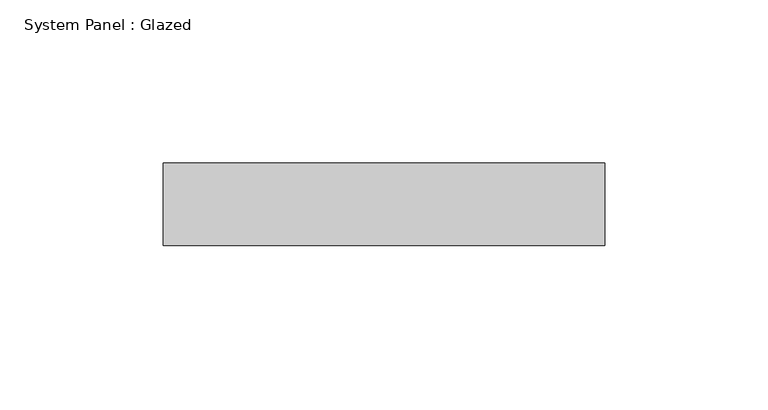
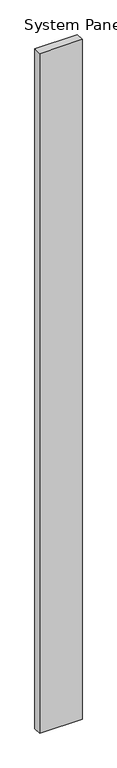
"""IFC4 building model written with IfcOpenShell, lengths in millimetres: plate geometry, System Panel : Glazed."""

from ifc_helpers import new_model, si_unit, origin, origin_with_axes, place, context, project, spatial, polyline, outline, extrude, source, transform, mapped, element, save


def system_panel_glazed_b538bb1a(model_context):
    return source(origin(), model_context, "Body", "SweptSolid", [
        extrude(outline(polyline([(67.7333333, 19.05), (-67.7333333, 19.05), (-67.7333333, 44.45), (67.7333333, 44.45), (67.7333333, 19.05)])), origin_with_axes(), (0.0, 0.0, 1.0), 2287.5875),
    ])


if __name__ == "__main__":
    model = new_model("IFC4")
    model_context = context("Model", 3, world=origin())
    ifc_project = project(units=[si_unit("LENGTHUNIT", "METRE", prefix="MILLI")], contexts=[model_context])
    site = spatial("IfcSite", under=ifc_project)
    building = spatial("IfcBuilding", under=site)
    placement = place(None, origin())
    system_panel_glazed_shape = system_panel_glazed_b538bb1a(model_context)
    element("IfcPlate", 1, ObjectType="System Panel : Glazed", at=placement, inside=building, context=model_context, shape_type="MappedRepresentation", body=[
        mapped(system_panel_glazed_shape, transform((0.0, 0.0, 0.0), x_axis=(1.0, 0.0, 0.0), y_axis=(0.0, 1.0, 0.0), z_axis=(0.0, 0.0, 1.0))),
    ])
    save(model, "model.ifc")

# Revit data of these elements
# Type "System Panel : Glazed"
#   Construction Type Id = "GSP4R"
#   Analytic Construction = "1/8 in Pilkington single glazing"
#   Visual Light Transmittance = 0.9
#   Solar Heat Gain Coefficient = 0.86
#   Heat Transfer Coefficient (U) = 1.18115 BTU/(h·ft²·°F)
#   Define Thermal Properties by = 1
# Element 1 (IfcPlate, "System Panel : Glazed")
#   Materials on its faces: "Glass"
# Materials
#   "Glass": class "Glass", colour RGB 0 128 192, transparency 0.75, Description = "Soda Lime Glass", Cost = 0
